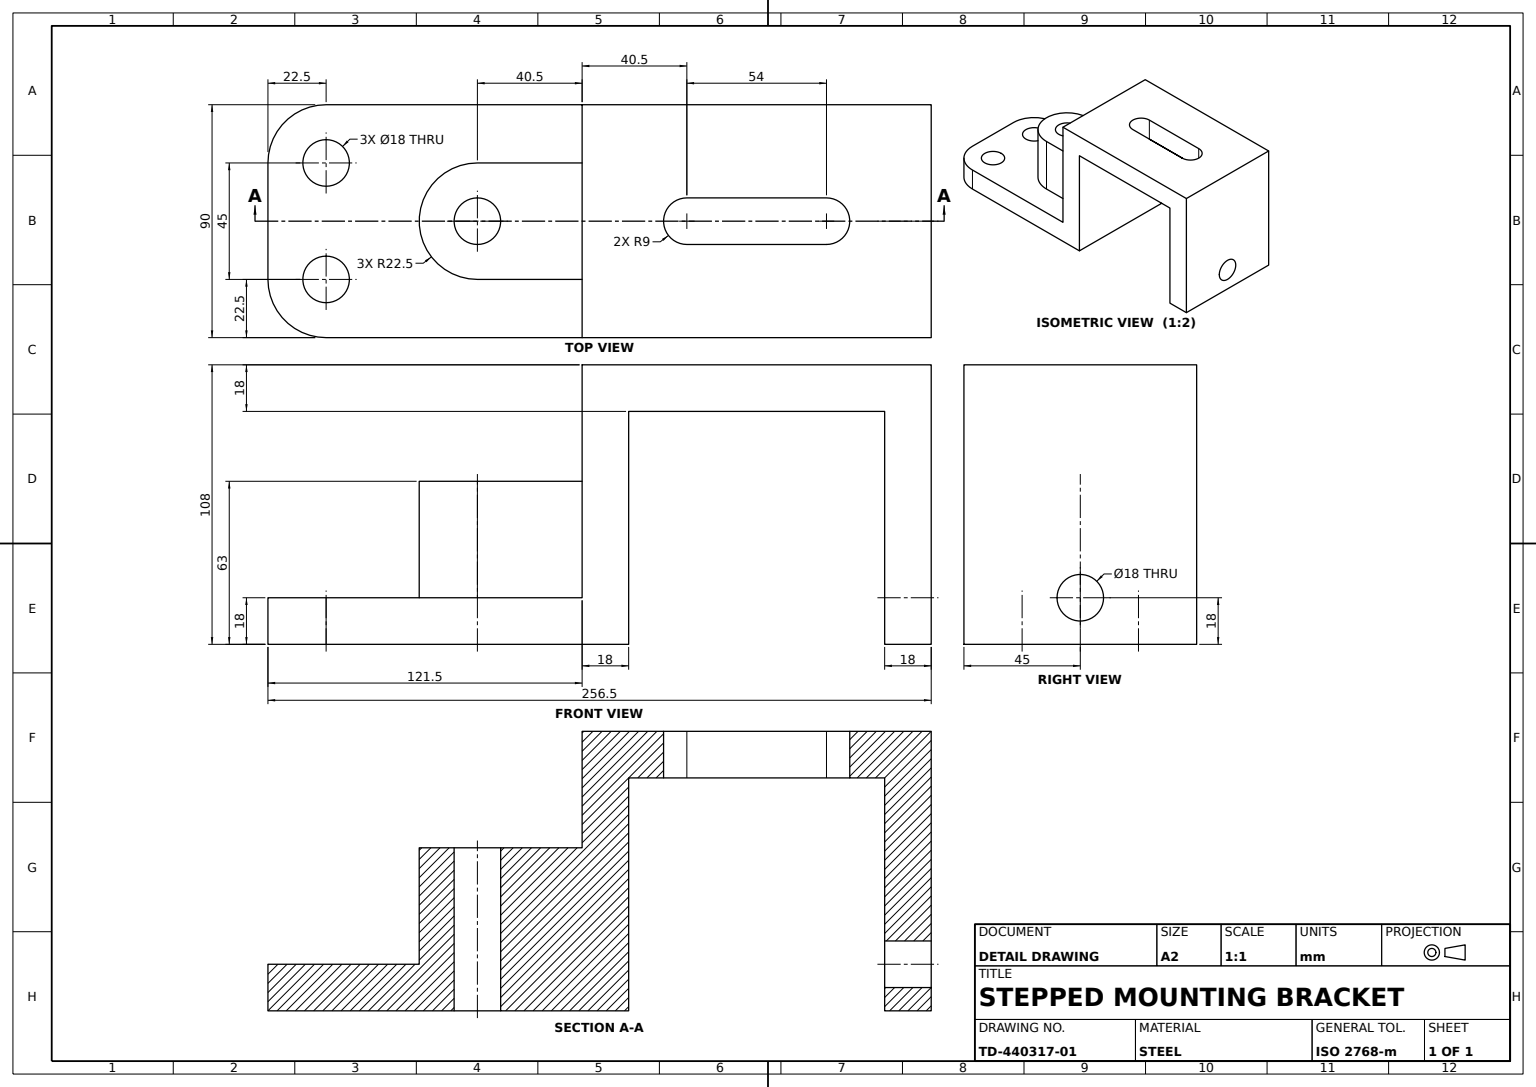
SolidWorks part; units mm, degrees
material "Plain Carbon Steel"
ref_plane "Front Plane" through (0, 0, 0) normal (0, 0, 1) x (1, 0, 0)
ref_plane "Top Plane" through (0, 0, 0) normal (0, 1, 0) x (1, 0, 0)
ref_plane "Right Plane" through (0, 0, 0) normal (1, 0, 0) x (0, 0, -1)
sketch "Bracket Profile Sketch" plane through (0, 0, 0) normal (0, 0, 1) x (1, 0, 0)
  line L0 (0, 165) -> (0, -165) construction
  line L1 (-244.75, 0) -> (244.75, 0) construction
  line L2 (0, 0) -> (0, 18)
  line L3 (0, 18) -> (121.5, 18)
  line L4 (121.5, 18) -> (121.5, 108)
  line L5 (121.5, 108) -> (256.5, 108)
  line L6 (256.5, 108) -> (256.5, 0)
  line L7 (256.5, 0) -> (238.5, 0)
  line L8 (238.5, 0) -> (238.5, 90)
  line L9 (238.5, 90) -> (139.5, 90)
  line L10 (139.5, 90) -> (139.5, 0)
  line L11 (139.5, 0) -> (0, 0)
  point P4 (0, 0)
  point P8 (0, 0)
  dimension "D1" = 99
  dimension "D2" = 18
  dimension "D3" = 135
  dimension "D4" = 108
  dimension "D5" = 18
  dimension "D6" = 121.5
  dimension "D7" = 18
extrude "Bracket Body" add sketch "Bracket Profile Sketch" along normal mid plane 90
sketch "Top Slot Sketch" plane through (0, 108, 0) normal (0, 1, 0) x (1, 0, 0)
  line L0 (162, 0) -> (216, 0) construction
  line L1 (162, 9) -> (216, 9)
  line L2 (162, -9) -> (216, -9)
  line L3 (256.5, 45) -> (121.5, 45) construction
  line L4 (189, 45) -> (189, -52.1725) construction
  arc A0 (162, 9) -> (162, -9) centre (162, 0) ccw
  arc A1 (216, -9) -> (216, 9) centre (216, 0) ccw
  point P2 (189, 0)
  point P12 (153, 0)
  point P13 (225, 0)
  dimension "D1" = 18
  dimension "D2" = 72
extrude "Top Slot 18x72" cut sketch "Top Slot Sketch" against normal mid plane 90
sketch "Pivot Boss Sketch" plane through (0, 18, 0) normal (0, 1, 0) x (1, 0, 0)
  line L0 (81, 0) -> (-81, 0) construction
  line L2 (81, 45) -> (81, -64.8975) construction
  line L3 (121.5, 45) -> (0, 45) construction
  line L4 (121.5, -45) -> (121.5, 45) construction
  line L5 (81, 22.5) -> (121.5, 22.5)
  line L6 (121.5, -45) -> (121.5, 45) construction
  line L7 (81, -22.5) -> (121.5, -22.5)
  line L8 (121.5, 22.5) -> (121.5, -22.5)
  arc A0 (81, 22.5) -> (81, -22.5) centre (81, 0) ccw
  point P4 (0, 0)
  dimension "D2" = 45
  dimension "D1" = 40.5
extrude "Pivot Boss" add sketch "Pivot Boss Sketch" along normal blind 45
sketch "Pivot Bore Sketch" plane through (0, 63, 0) normal (0, 1, 0) x (1, 0, 0)
  circle A0 centre (81, 0) radius 9
  dimension "D1" = 18
extrude "Pivot Bore Ø18" cut sketch "Pivot Bore Sketch" against normal blind 72 contours A0
fillet "Flange Corner Fillets R22.5" radius 22.5 2 edges at (0, 9, -45) (0, 9, 45)
sketch "Flange Holes Sketch" plane through (0, 18, 0) normal (0, 1, 0) x (1, 0, 0)
  circle A0 centre (22.5, 22.5) radius 9
  circle A1 centre (22.5, -22.5) radius 9
  dimension "D1" = 18
  dimension "D2" = 18
extrude "Flange Holes 2xØ18" cut sketch "Flange Holes Sketch" against normal blind 72
sketch "Side Hole Sketch" plane through (256.5, 0, 0) normal (1, 0, 0) x (0, 0, -1)
  line L0 (0, 0) -> (0, 109.6086) construction
  line L1 (-45, 0) -> (45, 0) construction
  circle A0 centre (0, 18) radius 9
  dimension "D2" = 18
  dimension "D1" = 18
  dimension "D3" = 109.6086
extrude "Side Hole Ø18" cut sketch "Side Hole Sketch" against normal blind 72
